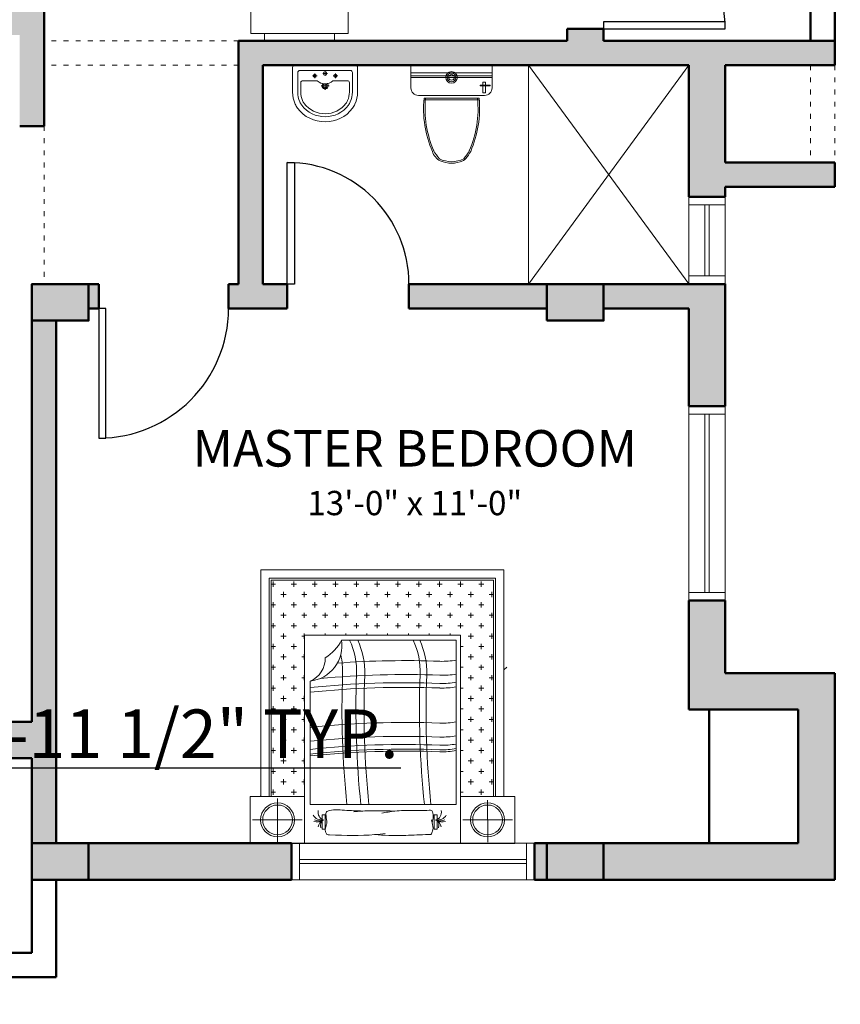
# Model space of a CAD drawing. Units: inches. Extents: x 375 to 1122, y 27 to 1069.
# Tile 67 of 155: x 788 to 990, y 157 to 400. Entities that reach past the tile are written whole.
import ezdxf

# ---------------------------------------------------------------- set-up
doc = ezdxf.new("R2010")
doc.units = ezdxf.units.IN
doc.linetypes.add('ACAD_ISO03W100', pattern=[30, 12, -18])
for name, color, linetype, lineweight in [('A-ANNO-DIMS', 2, 'Continuous', 18), ('A-AREA-IDEN', 7, 'Continuous', 18), ('A-COLS-PATT', 10, 'Continuous', 13), ('A-EQPM', 55, 'Continuous', 18), ('A-FLOR-FIXT', 55, 'Continuous', 18), ('A-WALL-OVHD', 77, 'ACAD_ISO03W100', 18), ('A-WALL-PATT', 252, 'Continuous', 13), ('Columns', 10, 'Continuous', 50), ('Doors', 150, 'Continuous', 25), ('Furniture', 30, 'Continuous', 18), ('Shower Areas', 53, 'Continuous', 18), ('Walls', 250, 'Continuous', 50), ('Windows', 122, 'Continuous', 18)]:
    doc.layers.add(name, color=color, linetype=linetype, lineweight=lineweight)
doc.styles.get("Standard").update_dxf_attribs({"font": 'arial.ttf'})
doc.dimstyles.new('ISO-25', dxfattribs={"dimtxt": 12, "dimasz": 2.5, "dimexe": 1.5, "dimexo": 1.5, "dimtad": 1, "dimdec": 1, "dimlunit": 3, "dimtxsty": 'Standard', "dimblk": 'ARCHTICK', "dimcen": 2.5, "dimadec": 0, "dimazin": 0, "dimtfac": 1, "dimtdec": 1, "dimtmove": 0, "dimatfit": 3, "dimfxl": 1.5, "dimfxlon": 1, "dimarcsym": 0})

# ---------------------------------------------------------------- blocks, each defined once
blk = doc.blocks.new('*U2')
for p, q in [((0, 0), (0, 4)), ((32, 0), (32, 4))]:
    blk.add_line(p, q)
blk.add_lwpolyline([(0, 0), (0, -32), (1.75, -32), (1.75, 0)], close=True)
blk.add_arc((0, 0), 32, 270, 0)
blk = doc.blocks.new('*U3')
for p, q in [((0, 0), (0, -4)), ((30, 0), (30, -4))]:
    blk.add_line(p, q)
blk.add_lwpolyline([(0, 0), (0, 30), (1.75, 30), (1.75, 0)], close=True)
blk.add_arc((0, 0), 30, 0, 90)
blk = doc.blocks.new('*U13')
for p, q in [((-30, 0), (-30, -4)), ((0, 0), (0, -4))]:
    blk.add_line(p, q)
blk.add_lwpolyline([(0, 0), (0, 30), (-1.75, 30), (-1.75, 0)], close=True)
blk.add_arc((0, 0), 30, 90, 180)
blk = doc.blocks.new('A$C52B64FF5')
for p, q in [((0.5216, 2.6276), (0, 2.6276)), ((0, 2.6276), (0, 2.1776)), ((0.2616, 2.4026), (0.2616, 2.6161)), ((0.5216, 2.1776), (0.5216, 2.6276)), ((2.0216, 2.6276), (0.5216, 2.6276)), ((0.5216, 2.6276), (0.5216, 0.6276)), ((2.5432, 2.6276), (2.0216, 2.6276)), ((2.0216, 0.6276), (2.0216, 2.6276)), ((2.0216, 2.6276), (2.0216, 2.1776)), ((2.2816, 2.4026), (2.2816, 2.6161)), ((2.5432, 2.1776), (2.5432, 2.6276)), ((0.721, 2.4927), (0.6917, 2.4927)), ((0.6917, 2.4927), (0.6917, 2.3531)), ((0.721, 2.3531), (0.721, 2.4927)), ((1.767, 2.3531), (1.767, 2.4927)), ((1.767, 2.4927), (1.7964, 2.4927)), ((1.7964, 2.4927), (1.7964, 2.3531)), ((0.2632, 2.4026), (0.0233, 2.4026)), ((0.0233, 2.4026), (0.4999, 2.4026)), ((0.2632, 2.1952), (0.2632, 2.4026)), ((2.5199, 2.4026), (2.0434, 2.4026)), ((2.2801, 2.2128), (2.2801, 2.4026)), ((2.2801, 2.4026), (2.5199, 2.4026)), ((0.6917, 2.3531), (0.721, 2.3531)), ((1.7964, 2.3531), (1.767, 2.3531)), ((0, 2.1776), (0.5216, 2.1776)), ((0.093, 2.1776), (0.1008, 2.1698)), ((0.1008, 0), (0.1008, 2.1776)), ((0.1808, 0.08), (0.1808, 2.1776)), ((0.2008, 0.1), (0.2008, 2.1776)), ((0.5751, 1.0685), (0.5751, 2.2541)), ((0.5751, 2.2541), (1.9782, 2.2541)), ((1.9782, 2.2541), (1.9782, 0.6749)), ((2.5432, 2.1776), (2.0216, 2.1776)), ((2.0216, 2.1776), (2.5432, 2.1776)), ((2.3374, 2.1776), (2.3374, 0.1)), ((2.3574, 2.1776), (2.3574, 0.08)), ((2.4374, 2.1776), (2.4374, 0)), ((0.2008, 2.136), (0.2447, 2.136)), ((0.2197, 2.111), (0.2197, 2.161)), ((0.3947, 2.136), (0.4447, 2.136)), ((0.4197, 2.111), (0.4197, 2.161)), ((2.0216, 2.136), (2.0447, 2.136)), ((2.1947, 2.136), (2.2447, 2.136)), ((2.2197, 2.111), (2.2197, 2.161)), ((0.2947, 2.036), (0.3447, 2.036)), ((0.3197, 2.011), (0.3197, 2.061)), ((0.4947, 2.036), (0.5216, 2.036)), ((0.5197, 2.011), (0.5197, 2.061)), ((2.0947, 2.036), (2.1447, 2.036)), ((2.1197, 2.011), (2.1197, 2.061)), ((2.2947, 2.036), (2.3374, 2.036)), ((2.3197, 2.011), (2.3197, 2.061)), ((0.2008, 1.936), (0.2447, 1.936)), ((0.2197, 1.911), (0.2197, 1.961)), ((0.3947, 1.936), (0.4447, 1.936)), ((0.4197, 1.911), (0.4197, 1.961)), ((2.0216, 1.936), (2.0447, 1.936)), ((2.1947, 1.936), (2.2447, 1.936)), ((2.2197, 1.911), (2.2197, 1.961)), ((0.2947, 1.836), (0.3447, 1.836)), ((0.3197, 1.811), (0.3197, 1.861)), ((0.4947, 1.836), (0.5216, 1.836)), ((0.5197, 1.811), (0.5197, 1.861)), ((2.0947, 1.836), (2.1447, 1.836)), ((2.1197, 1.811), (2.1197, 1.861)), ((2.2947, 1.836), (2.3374, 1.836)), ((2.3197, 1.811), (2.3197, 1.861)), ((0.2008, 1.736), (0.2447, 1.736)), ((0.2197, 1.711), (0.2197, 1.761)), ((0.3947, 1.736), (0.4447, 1.736)), ((0.4197, 1.711), (0.4197, 1.761)), ((2.0216, 1.736), (2.0447, 1.736)), ((2.1947, 1.736), (2.2447, 1.736)), ((2.2197, 1.711), (2.2197, 1.761)), ((0.2947, 1.636), (0.3447, 1.636)), ((0.3197, 1.611), (0.3197, 1.661)), ((0.4947, 1.636), (0.5216, 1.636)), ((0.5197, 1.611), (0.5197, 1.661)), ((2.0947, 1.636), (2.1447, 1.636)), ((2.1197, 1.611), (2.1197, 1.661)), ((2.2947, 1.636), (2.3374, 1.636)), ((2.3197, 1.611), (2.3197, 1.661)), ((0.2008, 1.536), (0.2447, 1.536)), ((0.2197, 1.511), (0.2197, 1.561)), ((0.3947, 1.536), (0.4447, 1.536)), ((0.4197, 1.511), (0.4197, 1.561)), ((2.0216, 1.536), (2.0447, 1.536)), ((2.1947, 1.536), (2.2447, 1.536)), ((2.2197, 1.511), (2.2197, 1.561)), ((0.2947, 1.436), (0.3447, 1.436)), ((0.3197, 1.411), (0.3197, 1.461)), ((0.4947, 1.436), (0.5216, 1.436)), ((0.5197, 1.411), (0.5197, 1.461)), ((2.0947, 1.436), (2.1447, 1.436)), ((2.1197, 1.411), (2.1197, 1.461)), ((2.2947, 1.436), (2.3374, 1.436)), ((2.3197, 1.411), (2.3197, 1.461)), ((0.2008, 1.336), (0.2447, 1.336)), ((0.2197, 1.311), (0.2197, 1.361)), ((0.3947, 1.336), (0.4447, 1.336)), ((0.4197, 1.311), (0.4197, 1.361)), ((2.0216, 1.336), (2.0447, 1.336)), ((2.1947, 1.336), (2.2447, 1.336)), ((2.2197, 1.311), (2.2197, 1.361)), ((0.2947, 1.236), (0.3447, 1.236)), ((0.3197, 1.211), (0.3197, 1.261)), ((0.4947, 1.236), (0.5216, 1.236)), ((0.5197, 1.211), (0.5197, 1.261)), ((2.0947, 1.236), (2.1447, 1.236)), ((2.1197, 1.211), (2.1197, 1.261)), ((2.2947, 1.236), (2.3374, 1.236)), ((2.3197, 1.211), (2.3197, 1.261)), ((0.2008, 1.136), (0.2447, 1.136)), ((0.2197, 1.111), (0.2197, 1.161)), ((0.3947, 1.136), (0.4447, 1.136)), ((0.4197, 1.111), (0.4197, 1.161)), ((2.0216, 1.136), (2.0447, 1.136)), ((2.1947, 1.136), (2.2447, 1.136)), ((2.2197, 1.111), (2.2197, 1.161)), ((0.3197, 1.011), (0.3197, 1.061)), ((0.5197, 1.011), (0.5197, 1.061)), ((2.1197, 1.011), (2.1197, 1.061)), ((2.3197, 1.011), (2.3197, 1.061)), ((0.2197, 0.911), (0.2197, 0.961)), ((0.2947, 1.036), (0.3447, 1.036)), ((0.4197, 0.911), (0.4197, 0.961)), ((0.4947, 1.036), (0.5216, 1.036)), ((2.0947, 1.036), (2.1447, 1.036)), ((2.2197, 0.911), (2.2197, 0.961)), ((2.2947, 1.036), (2.3374, 1.036)), ((2.4374, 0.9617), (2.4642, 0.935)), ((0.2008, 0.936), (0.2447, 0.936)), ((0.3197, 0.811), (0.3197, 0.861)), ((0.3947, 0.936), (0.4447, 0.936)), ((0.5197, 0.811), (0.5197, 0.861)), ((2.0216, 0.936), (2.0447, 0.936)), ((2.1197, 0.811), (2.1197, 0.861)), ((2.1947, 0.936), (2.2447, 0.936)), ((2.3197, 0.811), (2.3197, 0.861)), ((0.2197, 0.711), (0.2197, 0.761)), ((0.2947, 0.836), (0.3447, 0.836)), ((0.4197, 0.711), (0.4197, 0.761)), ((0.4947, 0.836), (0.5216, 0.836)), ((2.0947, 0.836), (2.1447, 0.836)), ((2.2197, 0.711), (2.2197, 0.761)), ((2.2947, 0.836), (2.3374, 0.836)), ((0.2008, 0.736), (0.2447, 0.736)), ((0.3947, 0.736), (0.4447, 0.736)), ((1.9782, 0.6749), (0.8764, 0.6749)), ((2.0216, 0.736), (2.0447, 0.736)), ((2.1947, 0.736), (2.2447, 0.736)), ((0.2947, 0.636), (0.3447, 0.636)), ((0.3197, 0.611), (0.3197, 0.661)), ((0.4947, 0.636), (0.5216, 0.636)), ((0.5197, 0.611), (0.5197, 0.661)), ((0.5216, 0.6276), (2.0216, 0.6276)), ((0.7197, 0.611), (0.7197, 0.6276)), ((0.9197, 0.611), (0.9197, 0.6276)), ((1.1197, 0.611), (1.1197, 0.6276)), ((1.3197, 0.611), (1.3197, 0.6276)), ((1.5197, 0.611), (1.5197, 0.6276)), ((1.7197, 0.611), (1.7197, 0.6276)), ((1.9197, 0.611), (1.9197, 0.6276)), ((2.0947, 0.636), (2.1447, 0.636)), ((2.1197, 0.611), (2.1197, 0.661)), ((2.2947, 0.636), (2.3374, 0.636)), ((2.3197, 0.611), (2.3197, 0.661)), ((0.2008, 0.536), (0.2447, 0.536)), ((0.2197, 0.511), (0.2197, 0.561)), ((0.3947, 0.536), (0.4447, 0.536)), ((0.4197, 0.511), (0.4197, 0.561)), ((0.5947, 0.536), (0.6447, 0.536)), ((0.6197, 0.511), (0.6197, 0.561)), ((0.7947, 0.536), (0.8447, 0.536)), ((0.8197, 0.511), (0.8197, 0.561)), ((0.9947, 0.536), (1.0447, 0.536)), ((1.0197, 0.511), (1.0197, 0.561)), ((1.1947, 0.536), (1.2447, 0.536)), ((1.2197, 0.511), (1.2197, 0.561)), ((1.3947, 0.536), (1.4447, 0.536)), ((1.4197, 0.511), (1.4197, 0.561)), ((1.5947, 0.536), (1.6447, 0.536)), ((1.6197, 0.511), (1.6197, 0.561)), ((1.7947, 0.536), (1.8447, 0.536)), ((1.8197, 0.511), (1.8197, 0.561)), ((1.9947, 0.536), (2.0447, 0.536)), ((2.0197, 0.511), (2.0197, 0.561)), ((2.1947, 0.536), (2.2447, 0.536)), ((2.2197, 0.511), (2.2197, 0.561)), ((0.2947, 0.436), (0.3447, 0.436)), ((0.3197, 0.411), (0.3197, 0.461)), ((0.4947, 0.436), (0.5447, 0.436)), ((0.5197, 0.411), (0.5197, 0.461)), ((0.6947, 0.436), (0.7447, 0.436)), ((0.7197, 0.411), (0.7197, 0.461)), ((0.8947, 0.436), (0.9447, 0.436)), ((0.9197, 0.411), (0.9197, 0.461)), ((1.0947, 0.436), (1.1447, 0.436)), ((1.1197, 0.411), (1.1197, 0.461)), ((1.2947, 0.436), (1.3447, 0.436)), ((1.3197, 0.411), (1.3197, 0.461)), ((1.4947, 0.436), (1.5447, 0.436)), ((1.5197, 0.411), (1.5197, 0.461)), ((1.6947, 0.436), (1.7447, 0.436)), ((1.7197, 0.411), (1.7197, 0.461)), ((1.8947, 0.436), (1.9447, 0.436)), ((1.9197, 0.411), (1.9197, 0.461)), ((2.0947, 0.436), (2.1447, 0.436)), ((2.1197, 0.411), (2.1197, 0.461)), ((2.2947, 0.436), (2.3374, 0.436)), ((2.3197, 0.411), (2.3197, 0.461)), ((0.2008, 0.336), (0.2447, 0.336)), ((0.2197, 0.311), (0.2197, 0.361)), ((0.3947, 0.336), (0.4447, 0.336)), ((0.4197, 0.311), (0.4197, 0.361)), ((0.5947, 0.336), (0.6447, 0.336)), ((0.6197, 0.311), (0.6197, 0.361)), ((0.7947, 0.336), (0.8447, 0.336)), ((0.8197, 0.311), (0.8197, 0.361)), ((0.9947, 0.336), (1.0447, 0.336)), ((1.0197, 0.311), (1.0197, 0.361)), ((1.1947, 0.336), (1.2447, 0.336)), ((1.2197, 0.311), (1.2197, 0.361)), ((1.3947, 0.336), (1.4447, 0.336)), ((1.4197, 0.311), (1.4197, 0.361)), ((1.5947, 0.336), (1.6447, 0.336)), ((1.6197, 0.311), (1.6197, 0.361)), ((1.7947, 0.336), (1.8447, 0.336)), ((1.8197, 0.311), (1.8197, 0.361)), ((1.9947, 0.336), (2.0447, 0.336)), ((2.0197, 0.311), (2.0197, 0.361)), ((2.1947, 0.336), (2.2447, 0.336)), ((2.2197, 0.311), (2.2197, 0.361)), ((0.2947, 0.236), (0.3447, 0.236)), ((0.3197, 0.211), (0.3197, 0.261)), ((0.4947, 0.236), (0.5447, 0.236)), ((0.5197, 0.211), (0.5197, 0.261)), ((0.6947, 0.236), (0.7447, 0.236)), ((0.7197, 0.211), (0.7197, 0.261)), ((0.8947, 0.236), (0.9447, 0.236)), ((0.9197, 0.211), (0.9197, 0.261)), ((1.0947, 0.236), (1.1447, 0.236)), ((1.1197, 0.211), (1.1197, 0.261)), ((1.2947, 0.236), (1.3447, 0.236)), ((1.3197, 0.211), (1.3197, 0.261)), ((1.4947, 0.236), (1.5447, 0.236)), ((1.5197, 0.211), (1.5197, 0.261)), ((1.6947, 0.236), (1.7447, 0.236)), ((1.7197, 0.211), (1.7197, 0.261)), ((1.8947, 0.236), (1.9447, 0.236)), ((1.9197, 0.211), (1.9197, 0.261)), ((2.0947, 0.236), (2.1447, 0.236)), ((2.1197, 0.211), (2.1197, 0.261)), ((2.2947, 0.236), (2.3374, 0.236)), ((2.3197, 0.211), (2.3197, 0.261)), ((0.2008, 0.136), (0.2447, 0.136)), ((2.3374, 0.1), (0.2008, 0.1)), ((0.2197, 0.111), (0.2197, 0.161)), ((0.3947, 0.136), (0.4447, 0.136)), ((0.4197, 0.111), (0.4197, 0.161)), ((0.5947, 0.136), (0.6447, 0.136)), ((0.6197, 0.111), (0.6197, 0.161)), ((0.7947, 0.136), (0.8447, 0.136)), ((0.8197, 0.111), (0.8197, 0.161)), ((0.9947, 0.136), (1.0447, 0.136)), ((1.0197, 0.111), (1.0197, 0.161)), ((1.1947, 0.136), (1.2447, 0.136)), ((1.2197, 0.111), (1.2197, 0.161)), ((1.3947, 0.136), (1.4447, 0.136)), ((1.4197, 0.111), (1.4197, 0.161)), ((1.5947, 0.136), (1.6447, 0.136)), ((1.6197, 0.111), (1.6197, 0.161)), ((1.7947, 0.136), (1.8447, 0.136)), ((1.8197, 0.111), (1.8197, 0.161)), ((1.9947, 0.136), (2.0447, 0.136)), ((2.0197, 0.111), (2.0197, 0.161)), ((2.1947, 0.136), (2.2447, 0.136)), ((2.2197, 0.111), (2.2197, 0.161)), ((2.4374, 0), (0.1008, 0)), ((2.3574, 0.08), (0.1808, 0.08))]:
    blk.add_line(p, q)
for centre, radius in [((0.2632, 2.4026), 0.1631), ((2.2801, 2.4026), 0.1631), ((0.2632, 2.4026), 0.1431), ((2.2801, 2.4026), 0.1431)]:
    blk.add_circle(centre, radius)
for centre, radius, start, end in [((0.7523, 2.4916), 0.1013, 192.77399, 239.2386), ((0.7566, 2.4523), 0.0808, 161.45592, 221.5545), ((1.7358, 2.4916), 0.1013, 300.7614, 347.22601), ((1.7315, 2.4523), 0.0808, 318.4455, 18.54408), ((0.6895, 2.3063), 0.098, 80.94857, 149.48786), ((0.6442, 2.3154), 0.1072, 59.2174, 107.24009), ((0.6646, 2.3215), 0.0913, 67.83977, 120.48585), ((0.7294, 2.33), 0.0776, 109.26419, 192.26691), ((1.7587, 2.33), 0.0776, 347.73309, 73.88358), ((1.7986, 2.3063), 0.098, 30.51214, 99.05143), ((1.8439, 2.3154), 0.1072, 72.75991, 120.7826), ((1.8235, 2.3215), 0.0913, 59.51415, 112.16023), ((9.7293, 1.3409), 8.8479, 174.07538, 182.16616), ((9.8633, 1.3409), 8.8479, 174.07538, 182.16616), ((9.9414, 1.3409), 8.8479, 174.07538, 182.16616), ((10.4736, 1.3409), 8.8479, 174.07538, 182.16616), ((10.5369, 1.3409), 8.8479, 174.07538, 182.16616), ((1.4884, 10.5889), 8.8479, 264.07538, 272.16616), ((1.4884, 10.5702), 8.8479, 264.07538, 272.16616), ((1.4884, 10.5256), 8.8479, 264.07538, 272.16616), ((1.85, 1.0282), 0.7196, 79.7409, 92.16616), ((1.85, 1.0096), 0.7196, 79.7409, 92.16616), ((1.4884, 10.4474), 8.8479, 264.07538, 272.16616), ((1.85, 0.965), 0.7196, 79.7409, 92.16616), ((1.85, 0.8868), 0.7196, 79.7409, 92.16616), ((1.4884, 10.3135), 8.8479, 264.07538, 272.16616), ((1.85, 0.7528), 0.7196, 79.7409, 92.16616), ((1.4884, 9.9764), 8.8479, 264.07538, 272.16616), ((1.4884, 9.9317), 8.8479, 264.07538, 272.16616), ((0.4865, 0.8516), 0.2343, 358.03681, 67.7864), ((0.5391, 0.7288), 0.3416, 350.92672, 83.95649), ((1.4884, 9.8536), 8.8479, 264.70583, 272.16616), ((1.85, 0.4158), 0.7196, 79.7409, 92.16616), ((1.85, 0.3711), 0.7196, 79.7409, 92.16616), ((0.1687, 0.9792), 0.7196, 346.86533, 2.16616), ((0.3027, 0.9792), 0.7196, 334.98359, 2.16616), ((0.3808, 0.9792), 0.7196, 334.98359, 2.16616), ((0.913, 0.9792), 0.7196, 334.98359, 2.16616), ((0.9763, 0.9792), 0.7196, 334.98359, 2.16616), ((1.85, 0.293), 0.7196, 79.7409, 92.16616), ((1.4884, 9.7196), 8.8479, 265.77852, 272.16616), ((1.85, 0.159), 0.7196, 79.7409, 92.16616), ((0.5285, 0.5098), 0.3852, 25.3912, 60.06861)]:
    blk.add_arc(centre, radius, start, end)
for points, knots in [([(0.7373, 2.4293), (0.7344, 2.4386), (0.7239, 2.472), (0.715, 2.518), (0.7414, 2.5459), (0.9088, 2.5514), (1.0864, 2.5586), (1.2642, 2.5365), (1.2976, 2.5323)], [0, 0, 0, 0, 0.0298664, 0.1071619, 0.1152509, 0.1416099, 0.5761797, 0.6768951, 0.6768951, 0.6768951, 0.6768951]), ([(1.1947, 2.5438), (1.2853, 2.549), (1.4483, 2.5585), (1.6283, 2.5432), (1.7179, 2.5437), (1.7351, 2.5438)], [0, 0, 0, 0, 0.2717358, 0.4891854, 0.5406465, 0.5406465, 0.5406465, 0.5406465]), ([(1.7351, 2.5438), (1.7416, 2.5321), (1.759, 2.5014), (1.7583, 2.4623), (1.7348, 2.3817), (1.7455, 2.4145), (1.7494, 2.4265)], [0, 0, 0, 0, 0.0383771, 0.1013156, 0.1484959, 0.1756343, 0.1756343, 0.1756343, 0.1756343]), ([(1.0802, 2.3175), (1.0225, 2.3155), (0.9099, 2.3116), (0.7905, 2.2985), (0.7234, 2.3279), (0.7309, 2.3766), (0.7348, 2.4091), (0.7373, 2.4293)], [0, 0, 0, 0, 0.1744349, 0.3406483, 0.347042, 0.3874998, 0.4538558, 0.4538558, 0.4538558, 0.4538558]), ([(1.7494, 2.4265), (1.7531, 2.4084), (1.7601, 2.3751), (1.7573, 2.3363), (1.7437, 2.3065), (1.6676, 2.315), (1.559, 2.3108), (1.4028, 2.3119), (1.305, 2.3301), (1.2633, 2.3378)], [0, 0, 0, 0, 0.0550284, 0.1011576, 0.1178362, 0.1437253, 0.3009935, 0.4726259, 0.6000038, 0.6000038, 0.6000038, 0.6000038]), ([(1.3748, 2.3178), (1.2947, 2.315), (1.1678, 2.3105), (1.0413, 2.32), (0.9946, 2.3235)], [0, 0, 0, 0, 0.2401688, 0.38052, 0.38052, 0.38052, 0.38052])]:
    blk.add_open_spline(points, degree=3, knots=knots)
blk = doc.blocks.new('A$C659B0DF6')
for p, q in [((17.35, 607.55), (17.35, 606.07)), ((21.05, 607.55), (17.35, 607.55)), ((21.05, 606.07), (21.05, 607.55)), ((24, 606.07), (0, 606.07)), ((0, 585.72), (0, 606.07)), ((24, 585.72), (24, 606.07)), ((24, 604.22), (0, 604.22)), ((24, 585.72), (0, 585.72)), ((3.37, 583.91), (3.37, 585.72)), ((20.63, 583.91), (20.63, 585.72)), ((3.37, 583.91), (20.63, 583.91))]:
    blk.add_line(p, q)
blk = doc.blocks.new('A$C00C51FE0')
at = {"ltscale": 2}
for p, q in [((1.85, 7.41), (18.15, 7.41)), ((16.79, 8.49), (3.21, 8.49)), ((16.79, 8.12), (3.21, 8.12)), ((0, 0), (0, 5.56)), ((0.5, 4.84), (0.5, 5.06)), ((0.5, 5.06), (2.91, 5.06)), ((1.59, 4.18), (1.59, 6.81)), ((1.59, 6.81), (2.25, 6.81)), ((2.25, 6.81), (2.25, 4.18)), ((2.91, 5.06), (2.91, 4.84)), ((20, 5.56), (20, 0)), ((20, 2.96), (0, 2.96)), ((20, 2.59), (0, 2.59)), ((2.91, 4.84), (0.5, 4.84)), ((2.25, 4.18), (1.59, 4.18)), ((20, 1.85), (0, 1.85)), ((20, 0), (0, 0))]:
    blk.add_line(p, q, dxfattribs=at)
for radius in [1.44, 1.07, 0.698]:
    blk.add_circle((10, 2.96), radius, dxfattribs=at)
for centre, radius, start, end in [((22.68, 10.69), 20.34, 142.816, 148.8373), ((22.68, 10.69), 19.97, 141.7352, 148.8373), ((7.96, 21.86), 1.85, 112.9199, 142.816), ((10, 17.03), 6.73, 63.5839, 116.4161), ((10, 17.03), 7.1, 67.0801, 112.9199), ((11.04, 20.15), 3.83, 16.1902, 63.2078), ((-2.68, 10.69), 19.97, 31.1627, 38.2648), ((29.69, 10.65), 26.6, 156.5869, 185.4494), ((29.69, 10.65), 26.23, 156.5869, 185.4494), ((-9.69, 10.65), 26.23, 354.5506, 23.4131), ((-9.69, 10.65), 26.6, 354.5506, 23.4131), ((1.85, 5.56), 1.85, 90, 180), ((18.15, 5.56), 1.85, 0, 90)]:
    blk.add_arc(centre, radius, start, end, dxfattribs=at)
blk = doc.blocks.new('WINDOW-48IN')
for p, q in [((2, 5), (46, 5)), ((2, 4), (46, 4))]:
    blk.add_line(p, q)
blk.add_lwpolyline([(48, 0), (0, 0), (0, 9), (48, 9)], close=True)
for points in [[(2, 0), (2, 9)], [(46, 9), (46, 0)]]:
    blk.add_lwpolyline(points)
blk = doc.blocks.new('WINDOW-21_5IN')
for p, q in [((4, 2), (4, 19.5)), ((5, 2), (5, 19.5))]:
    blk.add_line(p, q)
blk.add_lwpolyline([(0, 0), (9, 0), (9, 21.5), (0, 21.5)], close=True)
for points in [[(9, 19.5), (0, 19.5)], [(0, 2), (9, 2)]]:
    blk.add_lwpolyline(points)
blk = doc.blocks.new('WINDOW-60IN')
for p, q in [((58, 5), (2, 5)), ((58, 4), (2, 4))]:
    blk.add_line(p, q)
blk.add_lwpolyline([(60, 0), (0, 0), (0, 9), (60, 9)], close=True)
for points in [[(2, 0), (2, 9)], [(58, 9), (58, 0)]]:
    blk.add_lwpolyline(points)
blk = doc.blocks.new('LAVATORY-16IN')
for p, q in [((1.27, 7.37), (1.27, 12.19)), ((1.78, 12.7), (14.22, 12.7)), ((8, 11.37), (8, 12.51)), ((14.73, 12.19), (14.73, 7.37)), ((2.51, 10.16), (6.08, 10.16)), ((4.89, 11.37), (6.03, 11.37)), ((5.46, 10.79), (5.46, 11.94)), ((7.43, 11.94), (8.57, 11.94)), ((9.91, 10.16), (13.49, 10.16)), ((9.97, 11.37), (11.11, 11.37)), ((10.54, 10.79), (10.54, 11.94)), ((2.01, 7.37), (2.01, 9.65)), ((7.02, 8.89), (8.98, 8.89)), ((8, 7.91), (8, 9.4)), ((13.99, 9.65), (13.99, 7.37))]:
    blk.add_line(p, q)
blk.add_lwpolyline([(0.51, 13.97), (15.49, 13.97, -0.414214), (16, 13.46), (16, 7.37, -0.104704), (15.37, 4.36, -0.038376), (14.78, 3.36, -0.495903), (1.22, 3.36, -0.038376), (0.63, 4.36, -0.104704), (0, 7.37), (0, 13.46, -0.414214)], format="xyb", close=True)
for points in [[(1.27, 7.37, 0.102694), (1.78, 4.92, 0.037256), (2.25, 4.11, 0.085618)], [(2.01, 7.37, 0.101044), (2.44, 5.24, 0.036381), (2.84, 4.54, 0.084644)], [(13.16, 4.54, 0.036381), (13.56, 5.24, 0.101044), (13.99, 7.37, 0.11083)], [(13.75, 4.11, 0.037256), (14.22, 4.92, 0.102694), (14.73, 7.37, 0.111333)]]:
    blk.add_lwpolyline(points, format="xyb")
for centre, radius in [((8, 11.94), 0.444), ((5.46, 11.37), 0.381), ((10.54, 11.37), 0.381), ((8, 8.89), 0.508)]:
    blk.add_circle(centre, radius)
for centre, radius, start, end in [((1.78, 12.19), 0.508, 90, 180), ((14.22, 12.19), 0.508, 0, 90), ((2.51, 9.65), 0.508, 90, 180), ((7.99, 12.19), 2.79, 226.6581, 313.3419), ((13.49, 9.65), 0.508, 0, 90), ((8, 8.89), 0.762, 133.135, 47.0367), ((8, 8.52), 7.25, 217.471, 322.529), ((8, 8.52), 6.51, 217.6433, 322.3567)]:
    blk.add_arc(centre, radius, start, end)
blk = doc.blocks.new('COLUMN-14X9IN')
blk.add_lwpolyline([(0, 0), (14, 0), (14, 9), (0, 9)], close=True)
blk = doc.blocks.new('SHOWER-PAN-39_5X54IN')
for p, q in [((0, 0), (39.5, 54)), ((0, 54), (39.5, 0.05))]:
    blk.add_line(p, q)
blk.add_lwpolyline([(39.5, 54), (0, 54), (0, 0), (39.5, 0)], close=True)
blk = doc.blocks.new('_ArchTick')
at = {"color": 0, "linetype": 'ByBlock', "const_width": 0.15}
blk.add_lwpolyline([(-0.5, -0.5), (0.5, 0.5)], dxfattribs=at)
blk = doc.blocks.new('*D60')
at = {"layer": 'A-ANNO-DIMS', "color": 0, "lineweight": -2, "transparency": 16777216}
for p, q in [((684.39, 216.67), (684.39, 213.67)), ((767.77, 216.67), (767.77, 213.67)), ((684.39, 215.17), (767.77, 215.17)), ((767.77, 215.17), (882.02, 215.17))]:
    blk.add_line(p, q, dxfattribs=at)
at = {"layer": 'Defpoints', "color": 0, "transparency": 16777216}
for p in [(684.39, 232.35), (767.77, 232.35), (767.77, 215.17)]:
    blk.add_point(p, dxfattribs=at)
at = {"layer": 'A-ANNO-DIMS', "color": 0, "lineweight": -2, "transparency": 16777216, "xscale": 2.5, "yscale": 2.5, "zscale": 2.5, "rotation": 180}
blk.add_blockref('_ArchTick', (684.39, 215.17), dxfattribs=at)
at = {"layer": 'A-ANNO-DIMS', "color": 0, "lineweight": -2, "transparency": 16777216, "xscale": 2.5, "yscale": 2.5, "zscale": 2.5}
blk.add_blockref('_ArchTick', (767.77, 215.17), dxfattribs=at)
at = {"layer": 'A-ANNO-DIMS', "color": 0, "transparency": 16777216, "insert": (826.15, 222), "char_height": 12, "attachment_point": 5}
blk.add_mtext('6\'-11 1/2" TYP.', dxfattribs=at)
blk = doc.blocks.new('*D81')
at = {"layer": 'A-ANNO-DIMS', "color": 0, "lineweight": -2, "transparency": 16777216}
for p, q in [((444.51, 117.53), (444.51, 114.53)), ((989.01, 117.53), (989.01, 114.53)), ((444.51, 116.03), (989.01, 116.03))]:
    blk.add_line(p, q, dxfattribs=at)
at = {"layer": 'Defpoints', "color": 0, "transparency": 16777216}
for p in [(444.51, 187.53), (989.01, 187.53), (989.01, 116.03)]:
    blk.add_point(p, dxfattribs=at)
at = {"layer": 'A-ANNO-DIMS', "color": 0, "lineweight": -2, "transparency": 16777216, "xscale": 2.5, "yscale": 2.5, "zscale": 2.5, "rotation": 180}
blk.add_blockref('_ArchTick', (444.51, 116.03), dxfattribs=at)
at = {"layer": 'A-ANNO-DIMS', "color": 0, "lineweight": -2, "transparency": 16777216, "xscale": 2.5, "yscale": 2.5, "zscale": 2.5}
blk.add_blockref('_ArchTick', (989.01, 116.03), dxfattribs=at)
at = {"layer": 'A-ANNO-DIMS', "color": 0, "transparency": 16777216, "insert": (716.76, 122.86), "char_height": 12, "attachment_point": 5}
blk.add_mtext('45\'-4 1/2"', dxfattribs=at)
blk = doc.blocks.new('*D84')
at = {"layer": 'A-ANNO-DIMS', "color": 0, "lineweight": -2, "transparency": 16777216}
for p, q in [((845.01, 117.53), (845.01, 114.53)), ((950.01, 117.53), (950.01, 114.53)), ((845.01, 116.03), (950.01, 116.03))]:
    blk.add_line(p, q, dxfattribs=at)
at = {"layer": 'Defpoints', "color": 0, "transparency": 16777216}
for p in [(845.01, 814.53), (950.01, 814.53), (950.01, 116.03)]:
    blk.add_point(p, dxfattribs=at)
at = {"layer": 'A-ANNO-DIMS', "color": 0, "lineweight": -2, "transparency": 16777216, "xscale": 2.5, "yscale": 2.5, "zscale": 2.5, "rotation": 180}
blk.add_blockref('_ArchTick', (845.01, 116.03), dxfattribs=at)
at = {"layer": 'A-ANNO-DIMS', "color": 0, "lineweight": -2, "transparency": 16777216, "xscale": 2.5, "yscale": 2.5, "zscale": 2.5}
blk.add_blockref('_ArchTick', (950.01, 116.03), dxfattribs=at)
at = {"layer": 'A-ANNO-DIMS', "color": 0, "transparency": 16777216, "insert": (897.51, 122.78), "char_height": 12, "attachment_point": 5}
blk.add_mtext('8\'-9"', dxfattribs=at)
blk = doc.blocks.new('*D87')
at = {"layer": 'A-ANNO-DIMS', "color": 0, "lineweight": -2, "transparency": 16777216}
for p, q in [((794.01, 117.53), (794.01, 114.53)), ((884.01, 117.53), (884.01, 114.53)), ((794.01, 116.03), (884.01, 116.03))]:
    blk.add_line(p, q, dxfattribs=at)
at = {"layer": 'Defpoints', "color": 0, "transparency": 16777216}
for p in [(794.01, 583.53), (884.01, 583.53), (884.01, 116.03)]:
    blk.add_point(p, dxfattribs=at)
at = {"layer": 'A-ANNO-DIMS', "color": 0, "lineweight": -2, "transparency": 16777216, "xscale": 2.5, "yscale": 2.5, "zscale": 2.5, "rotation": 180}
blk.add_blockref('_ArchTick', (794.01, 116.03), dxfattribs=at)
at = {"layer": 'A-ANNO-DIMS', "color": 0, "lineweight": -2, "transparency": 16777216, "xscale": 2.5, "yscale": 2.5, "zscale": 2.5}
blk.add_blockref('_ArchTick', (884.01, 116.03), dxfattribs=at)
at = {"layer": 'A-ANNO-DIMS', "color": 0, "transparency": 16777216, "insert": (839.01, 122.78), "char_height": 12, "attachment_point": 5}
blk.add_mtext('7\'-6"', dxfattribs=at)
blk = doc.blocks.new('*D89')
at = {"layer": 'A-ANNO-DIMS', "color": 0, "lineweight": -2, "transparency": 16777216}
for p, q in [((863.01, 117.53), (863.01, 114.53)), ((923.01, 117.53), (923.01, 114.53)), ((863.01, 116.03), (923.01, 116.03))]:
    blk.add_line(p, q, dxfattribs=at)
at = {"layer": 'Defpoints', "color": 0, "transparency": 16777216}
for p in [(863.01, 574.53), (923.01, 574.53), (923.01, 116.03)]:
    blk.add_point(p, dxfattribs=at)
at = {"layer": 'A-ANNO-DIMS', "color": 0, "lineweight": -2, "transparency": 16777216, "xscale": 2.5, "yscale": 2.5, "zscale": 2.5, "rotation": 180}
blk.add_blockref('_ArchTick', (863.01, 116.03), dxfattribs=at)
at = {"layer": 'A-ANNO-DIMS', "color": 0, "lineweight": -2, "transparency": 16777216, "xscale": 2.5, "yscale": 2.5, "zscale": 2.5}
blk.add_blockref('_ArchTick', (923.01, 116.03), dxfattribs=at)
at = {"layer": 'A-ANNO-DIMS', "color": 0, "transparency": 16777216, "insert": (893.01, 122.78), "char_height": 12, "attachment_point": 5}
blk.add_mtext('5\'-0"', dxfattribs=at)

msp = doc.modelspace()

# ---------------------------------------------------------------- hatches: boundary and pattern name
at = {"layer": 'A-COLS-PATT'}
h = msp.add_hatch(color=256, dxfattribs=at)
h.dxf.hatch_style = 1
h.paths.add_polyline_path([(512.51, 982.53), (498.51, 982.53), (498.51, 973.53), (512.51, 973.53)])
h.paths.add_polyline_path([(666.51, 982.53), (652.51, 982.53), (652.51, 973.53), (666.51, 973.53)])
h.paths.add_polyline_path([(802.01, 982.53), (788.01, 982.53), (788.01, 973.53), (802.01, 973.53)])
h.paths.add_polyline_path([(932.01, 982.53), (918.01, 982.53), (918.01, 973.53), (932.01, 973.53)])
h.paths.add_polyline_path([(507.51, 841.53), (498.51, 841.53), (498.51, 827.53), (507.51, 827.53)])
h.paths.add_polyline_path([(666.51, 844.53), (652.51, 844.53), (652.51, 835.53), (666.51, 835.53)])
h.paths.add_polyline_path([(802.01, 814.53), (788.01, 814.53), (788.01, 805.53), (802.01, 805.53)])
h.paths.add_polyline_path([(932.01, 814.53), (918.01, 814.53), (918.01, 805.53), (932.01, 805.53)])
h.paths.add_polyline_path([(507.51, 719.53), (498.51, 719.53), (498.51, 705.53), (507.51, 705.53)])
h.paths.add_polyline_path([(731.01, 676.53), (722.01, 676.53), (722.01, 662.53), (731.01, 662.53)])
h.paths.add_polyline_path([(802.01, 676.53), (788.01, 676.53), (788.01, 667.53), (802.01, 667.53)])
h.paths.add_polyline_path([(932.01, 676.53), (918.01, 676.53), (918.01, 667.53), (932.01, 667.53)])
h.paths.add_polyline_path([(932.01, 583.53), (918.01, 583.53), (918.01, 574.53), (932.01, 574.53)])
h.paths.add_polyline_path([(868.01, 583.53), (854.01, 583.53), (854.01, 574.53), (868.01, 574.53)])
h.paths.add_polyline_path([(868.01, 502.53), (854.01, 502.53), (854.01, 493.53), (868.01, 493.53)])
h.paths.add_polyline_path([(932.01, 502.53), (918.01, 502.53), (918.01, 493.53), (932.01, 493.53)])
h.paths.add_polyline_path([(672.51, 592.03), (663.51, 592.03), (663.51, 578.03), (672.51, 578.03)])
h.paths.add_polyline_path([(512.51, 589.53), (498.51, 589.53), (498.51, 580.53), (512.51, 580.53)])
h.paths.add_polyline_path([(507.51, 464.53), (498.51, 464.53), (498.51, 450.53), (507.51, 450.53)])
h.paths.add_polyline_path([(731.01, 507.53), (722.01, 507.53), (722.01, 493.53), (731.01, 493.53)])
h.paths.add_polyline_path([(802.01, 502.53), (788.01, 502.53), (788.01, 493.53), (802.01, 493.53)])
h.paths.add_polyline_path([(507.51, 342.53), (498.51, 342.53), (498.51, 328.53), (507.51, 328.53)])
h.paths.add_polyline_path([(512.51, 196.53), (498.51, 196.53), (498.51, 187.53), (512.51, 187.53)])
h.paths.add_polyline_path([(666.51, 334.53), (652.51, 334.53), (652.51, 325.53), (666.51, 325.53)])
h.paths.add_polyline_path([(666.51, 196.53), (652.51, 196.53), (652.51, 187.53), (666.51, 187.53)])
h.paths.add_polyline_path([(805.01, 196.53), (791.01, 196.53), (791.01, 187.53), (805.01, 187.53)])
h.paths.add_polyline_path([(932.01, 196.53), (918.01, 196.53), (918.01, 187.53), (932.01, 187.53)])
h.paths.add_polyline_path([(932.01, 334.53), (918.01, 334.53), (918.01, 325.53), (932.01, 325.53)])
h.paths.add_polyline_path([(805.01, 334.53), (791.01, 334.53), (791.01, 325.53), (805.01, 325.53)])
at = {"layer": 'A-WALL-PATT'}
h = msp.add_hatch(color=256, dxfattribs=at)
h.dxf.hatch_style = 1
h.paths.add_polyline_path([(962.01, 388.53), (989.01, 388.53), (989.01, 394.53), (962.01, 394.53), (932.01, 394.53), (932.01, 397.53), (923.01, 397.53), (923.01, 394.53), (842.01, 394.53), (842.01, 334.53), (839.51, 334.53), (839.51, 328.53), (854.01, 328.53), (854.01, 334.53), (848.01, 334.53), (848.01, 388.53), (953.01, 388.53), (953.01, 356.08), (962.01, 356.08), (962.01, 358.55), (989.01, 358.55), (989.01, 364.55), (962.01, 364.55)])
h.paths.add_polyline_path([(989.01, 502.53), (932.01, 502.53), (932.01, 583.53), (932.01, 593.53), (923.01, 593.53), (923.01, 583.53), (854.01, 583.53), (854.01, 556.53), (863.01, 556.53), (863.01, 574.53), (923.01, 574.53), (923.01, 502.53), (863.01, 502.53), (863.01, 520.53), (854.01, 520.53), (854.01, 502.53), (773.01, 502.53), (773.01, 493.53), (788.01, 493.53), (788.01, 402.03), (722.01, 402.03), (722.01, 373.53), (728.01, 373.53), (728.01, 396.03), (788.01, 396.03), (788.01, 373.53), (794.01, 373.53), (794.01, 430.53), (814.01, 430.53), (814.01, 436.53), (794.01, 436.53), (794.01, 493.53), (923.01, 493.53), (923.01, 487.53), (932.01, 487.53), (932.01, 493.53), (983.01, 493.53), (983.01, 473.53), (989.01, 473.53)])
h.paths.add_polyline_path([(797.01, 325.53), (805.01, 325.53), (805.01, 328.53), (807.51, 328.53), (807.51, 334.53), (791.01, 334.53), (791.01, 226.53), (770.76, 226.53), (770.76, 217.53), (791.01, 217.53), (791.01, 187.53), (855.01, 187.53), (855.01, 196.53), (797.01, 196.53)])
h.paths.add_polyline_path([(989.01, 238.53), (962.01, 238.53), (962.01, 256.42), (953.01, 256.42), (953.01, 229.53), (980.01, 229.53), (980.01, 196.53), (915.01, 196.53), (915.01, 187.53), (989.01, 187.53)])
h.paths.add_polyline_path([(962.01, 334.53), (884.01, 334.53), (884.01, 328.53), (918.01, 328.53), (918.01, 325.53), (932.01, 325.53), (932.01, 328.53), (953.01, 328.53), (953.01, 304.42), (962.01, 304.42)])
h.paths.add_polyline_path([(606.51, 283.53), (609.51, 283.53), (609.51, 289.53), (600.51, 289.53), (600.51, 196.53), (578.51, 196.53), (578.51, 187.53), (606.51, 187.53), (606.51, 196.53)])
h.paths.add_polyline_path([(666.51, 292.53), (660.51, 292.53), (660.51, 289.53), (633.51, 289.53), (633.51, 283.53), (660.51, 283.53), (660.51, 196.53), (628.01, 196.53), (628.01, 187.53), (630.53, 187.53), (630.53, 160.53), (636.53, 160.53), (636.53, 187.53), (660.51, 187.53), (660.51, 160.53), (666.51, 160.53), (666.51, 217.53), (686.76, 217.53), (686.76, 226.53), (666.51, 226.53)])
h.paths.add_polyline_path([(480.51, 256.42), (471.51, 256.42), (471.51, 238.53), (444.51, 238.53), (444.51, 187.53), (518.51, 187.53), (518.51, 196.53), (453.51, 196.53), (453.51, 229.53), (480.51, 229.53)])
h.paths.add_polyline_path([(480.51, 328.53), (652.51, 328.53), (652.51, 325.53), (660.51, 325.53), (660.51, 322.53), (666.51, 322.53), (666.51, 334.53), (507.51, 334.53), (507.51, 360.53), (498.51, 360.53), (498.51, 334.53), (471.51, 334.53), (471.51, 304.42), (480.51, 304.42)])
h.paths.add_polyline_path([(507.51, 484.53), (498.51, 484.53), (498.51, 444.53), (507.51, 444.53), (507.51, 454.53), (621.51, 454.53), (621.51, 460.53), (507.51, 460.53)])
h.paths.add_polyline_path([(672.51, 604.53), (683.26, 604.53), (683.26, 613.53), (669.51, 613.53), (669.51, 649.53), (663.51, 649.53), (663.51, 589.53), (507.51, 589.53), (507.51, 613.53), (498.51, 613.53), (498.51, 556.53), (507.51, 556.53), (507.51, 580.53), (663.51, 580.53), (663.51, 520.53), (669.51, 520.53), (669.51, 556.53), (683.26, 556.53), (683.26, 565.53), (672.51, 565.53)])
h.paths.add_polyline_path([(731.01, 667.53), (734.01, 667.53), (734.01, 676.53), (728.01, 676.53), (728.01, 715.53), (657.51, 715.53), (657.51, 709.53), (663.51, 709.53), (663.51, 673.53), (669.51, 673.53), (669.51, 709.53), (722.01, 709.53), (722.01, 613.53), (704.76, 613.53), (704.76, 604.53), (722.01, 604.53), (722.01, 565.53), (704.76, 565.53), (704.76, 556.53), (722.01, 556.53), (722.01, 502.53), (722.01, 460.53), (669.51, 460.53), (669.51, 496.53), (663.51, 496.53), (663.51, 460.53), (657.51, 460.53), (657.51, 454.53), (728.01, 454.53), (728.01, 493.53), (734.01, 493.53), (734.01, 502.53), (731.01, 502.53)])
h.paths.add_polyline_path([(986.01, 718.53), (959.01, 718.53), (959.01, 727.53), (950.01, 727.53), (950.01, 709.53), (977.01, 709.53), (977.01, 676.53), (794.01, 676.53), (794.01, 805.53), (802.01, 805.53), (802.01, 808.53), (804.51, 808.53), (804.51, 814.53), (788.01, 814.53), (788.01, 774.03), (728.01, 774.03), (728.01, 796.53), (722.01, 796.53), (722.01, 768.03), (788.01, 768.03), (788.01, 676.53), (773.01, 676.53), (773.01, 667.53), (923.01, 667.53), (923.01, 657.53), (932.01, 657.53), (932.01, 667.53), (986.01, 667.53)])
h.paths.add_polyline_path([(621.51, 715.53), (507.51, 715.53), (507.51, 733.53), (498.51, 733.53), (498.51, 715.53), (498.51, 685.53), (507.51, 685.53), (507.51, 709.53), (621.51, 709.53)])
h.paths.add_polyline_path([(666.51, 847.03), (660.51, 847.03), (660.51, 844.53), (652.51, 844.53), (652.51, 841.53), (480.51, 841.53), (480.51, 859.53), (471.51, 859.53), (471.51, 835.53), (498.51, 835.53), (498.51, 817.53), (507.51, 817.53), (507.51, 835.53), (666.51, 835.53)])
h.paths.add_polyline_path([(480.51, 940.53), (453.51, 940.53), (453.51, 973.53), (518.51, 973.53), (518.51, 982.53), (444.51, 982.53), (444.51, 931.53), (471.51, 931.53), (471.51, 907.53), (480.51, 907.53)])
h.paths.add_polyline_path([(606.51, 982.53), (578.51, 982.53), (578.51, 973.53), (600.51, 973.53), (600.51, 880.53), (609.51, 880.53), (609.51, 886.53), (606.51, 886.53)])
h.paths.add_polyline_path([(666.51, 943.53), (686.76, 943.53), (686.76, 952.53), (666.51, 952.53), (666.51, 1009.53), (660.51, 1009.53), (660.51, 982.53), (636.53, 982.53), (636.53, 1009.53), (630.53, 1009.53), (630.53, 982.53), (628.01, 982.53), (628.01, 973.53), (660.51, 973.53), (660.51, 886.53), (633.51, 886.53), (633.51, 880.53), (660.51, 880.53), (660.51, 877.03), (666.51, 877.03)])
h.paths.add_polyline_path([(986.01, 874.53), (932.01, 874.53), (932.01, 877.53), (923.01, 877.53), (923.01, 874.53), (788.01, 874.53), (788.01, 868.53), (788.01, 844.53), (794.01, 844.53), (794.01, 868.53), (839.01, 868.53), (839.01, 814.53), (836.51, 814.53), (836.51, 808.53), (851.01, 808.53), (851.01, 814.53), (845.01, 814.53), (845.01, 868.53), (986.01, 868.53)])
h.paths.add_polyline_path([(959.01, 838.55), (986.01, 838.55), (986.01, 844.55), (959.01, 844.55), (959.01, 847.03), (950.01, 847.03), (950.01, 814.53), (881.01, 814.53), (881.01, 808.53), (918.01, 808.53), (918.01, 805.53), (932.01, 805.53), (932.01, 808.53), (950.01, 808.53), (950.01, 793.53), (959.01, 793.53)])
h.paths.add_polyline_path([(986.01, 982.53), (899.01, 982.53), (899.01, 973.53), (923.01, 973.53), (923.01, 967.53), (932.01, 967.53), (932.01, 973.53), (980.01, 973.53), (980.01, 953.53), (986.01, 953.53)])
h.paths.add_polyline_path([(851.01, 982.53), (788.01, 982.53), (788.01, 952.53), (770.76, 952.53), (770.76, 943.53), (788.01, 943.53), (788.01, 910.53), (814.01, 910.53), (814.01, 916.53), (794.01, 916.53), (794.01, 973.53), (851.01, 973.53)])

# ---------------------------------------------------------------- linework, layer by layer
at = {"layer": 'A-WALL-OVHD', "ltscale": 0.1}
for p, q in [((842.01, 394.53), (794.01, 394.53)), ((842.01, 388.53), (794.01, 388.53)), ((983.01, 388.53), (983.01, 364.55)), ((989.01, 388.53), (989.01, 364.55)), ((794.01, 373.53), (794.01, 334.53))]:
    msp.add_line(p, q, dxfattribs=at)
at = {"layer": 'Walls'}
for p, q in [((989.01, 394.53), (989.01, 502.53)), ((983.01, 394.53), (983.01, 493.53)), ((794.01, 373.53), (794.01, 430.53)), ((923.01, 394.53), (923.01, 397.53)), ((932.01, 397.53), (923.01, 397.53)), ((932.01, 394.53), (932.01, 397.53)), ((842.01, 334.53), (842.01, 394.53)), ((923.01, 394.53), (842.01, 394.53)), ((962.01, 394.53), (932.01, 394.53)), ((989.01, 394.53), (962.01, 394.53)), ((989.01, 394.53), (989.01, 388.53)), ((953.01, 388.53), (848.01, 388.53)), ((848.01, 334.53), (848.01, 388.53)), ((953.01, 356.08), (953.01, 388.53)), ((962.01, 364.55), (962.01, 388.53)), ((989.01, 388.53), (962.01, 388.53)), ((962.01, 364.55), (962.01, 388.53)), ((788.01, 373.53), (794.01, 373.53)), ((989.01, 364.55), (962.01, 364.55)), ((989.01, 358.55), (989.01, 364.55)), ((962.01, 358.55), (989.01, 358.55)), ((962.01, 356.08), (962.01, 358.55)), ((962.01, 356.08), (953.01, 356.08)), ((791.01, 334.53), (791.01, 226.53)), ((791.01, 334.53), (807.51, 334.53)), ((807.51, 334.53), (807.51, 328.53)), ((839.51, 334.53), (839.51, 328.53)), ((839.51, 334.53), (842.01, 334.53)), ((848.01, 334.53), (854.01, 334.53)), ((854.01, 334.53), (854.01, 328.53)), ((884.01, 334.53), (884.01, 328.53)), ((884.01, 334.53), (962.01, 334.53)), ((953.01, 334.53), (953.01, 334.58)), ((962.01, 334.53), (962.01, 334.58)), ((962.01, 334.53), (962.01, 304.42)), ((805.01, 328.53), (807.51, 328.53)), ((805.01, 325.53), (805.01, 328.53)), ((839.51, 328.53), (854.01, 328.53)), ((884.01, 328.53), (918.01, 328.53)), ((918.01, 328.53), (918.01, 325.53)), ((932.01, 328.53), (953.01, 328.53)), ((932.01, 325.53), (932.01, 328.53)), ((953.01, 328.53), (953.01, 304.42)), ((797.01, 325.53), (797.01, 196.53)), ((797.01, 325.53), (805.01, 325.53)), ((918.01, 325.53), (932.01, 325.53)), ((953.01, 304.42), (962.01, 304.42)), ((953.01, 256.42), (962.01, 256.42)), ((953.01, 256.42), (953.01, 229.53)), ((962.01, 256.42), (962.01, 238.53)), ((989.01, 238.53), (962.01, 238.53)), ((989.01, 187.53), (989.01, 238.53)), ((980.01, 229.53), (953.01, 229.53)), ((958.01, 196.53), (958.01, 229.53)), ((980.01, 196.53), (980.01, 229.53)), ((791.01, 226.53), (770.76, 226.53)), ((791.01, 217.53), (770.76, 217.53)), ((791.01, 217.53), (791.01, 169.53)), ((797.01, 196.53), (855.01, 196.53)), ((855.01, 187.53), (855.01, 196.53)), ((915.01, 187.53), (915.01, 196.53)), ((915.01, 196.53), (980.01, 196.53)), ((791.01, 187.53), (855.01, 187.53)), ((797.01, 187.53), (797.01, 163.53)), ((915.01, 187.53), (989.01, 187.53)), ((791.01, 169.53), (666.51, 169.53)), ((797.01, 163.53), (666.51, 163.53))]:
    msp.add_line(p, q, dxfattribs=at)

# ---------------------------------------------------------------- block references
at = {"layer": 'A-EQPM'}
msp.add_blockref('A$C659B0DF6', (845.01, -189.39), dxfattribs=at)
at = {"layer": 'A-FLOR-FIXT'}
msp.add_blockref('LAVATORY-16IN', (855.32, 374.56), dxfattribs=at)
at = {"layer": 'A-FLOR-FIXT', "rotation": 180}
msp.add_blockref('A$C00C51FE0', (904.51, 388.5), dxfattribs=at)
at = {"layer": 'Columns'}
for p in [(791.01, 325.53), (918.01, 325.53), (918.01, 187.53)]:
    msp.add_blockref('COLUMN-14X9IN', p, dxfattribs=at)
at = {"layer": 'Columns', "extrusion": (0, 0, -1), "zscale": -1, "rotation": 180}
msp.add_blockref('COLUMN-14X9IN', (-791.01, 196.53), dxfattribs=at)
at = {"layer": 'Doors', "rotation": 270}
msp.add_blockref('*U13', (932.01, 397.53), dxfattribs=at)
at = {"layer": 'Doors'}
for name, p in [('*U3', (854.01, 334.53)), ('*U2', (807.51, 328.53))]:
    msp.add_blockref(name, p, dxfattribs=at)
at = {"layer": 'Furniture', "xscale": -25.67804170018038, "yscale": 25.67804170018038, "zscale": 25.67804170018038, "rotation": 180}
msp.add_blockref('A$C52B64FF5', (844.85, 264), dxfattribs=at)
at = {"layer": 'Shower Areas'}
msp.add_blockref('SHOWER-PAN-39_5X54IN', (913.51, 334.53), dxfattribs=at)
at = {"layer": 'Windows'}
for name, p in [('WINDOW-21_5IN', (953.01, 334.58)), ('WINDOW-60IN', (855.01, 187.53))]:
    msp.add_blockref(name, p, dxfattribs=at)
at = {"layer": 'Windows', "rotation": 270}
msp.add_blockref('WINDOW-48IN', (953.01, 304.42), dxfattribs=at)

# ---------------------------------------------------------------- texts
at = {"layer": 'A-AREA-IDEN', "insert": (823.51, 298.5), "char_height": 12, "attachment_point": 1}
msp.add_mtext_dynamic_manual_height_columns('\\pxqc;{\\fArial|b1|i0|c0|p34;\\H0.75x;MASTER BEDROOM\\H1.33333x;\\P\\fArial|b0|i0|c0|p34;\\H0.5x;13\'-0" x 11\'-0"}', width=123.8705, gutter_width=12.5, heights=[0], dxfattribs=at)

# ---------------------------------------------------------------- dimensions: what is measured, and where the dimension line sits
at = {"layer": 'A-ANNO-DIMS'}
for base, p1, p2, picture, middle in [((950.01, 116.03), (845.01, 814.53), (950.01, 814.53), '*D84', (897.51, 122.78)), ((884.01, 116.03), (794.01, 583.53), (884.01, 583.53), '*D87', (839.01, 122.78)), ((923.01, 116.03), (863.01, 574.53), (923.01, 574.53), '*D89', (893.01, 122.78)), ((989.01, 116.03), (444.51, 187.53), (989.01, 187.53), '*D81', (716.76, 122.86))]:
    dim = msp.add_linear_dim(base=base, p1=p1, p2=p2, dimstyle='ISO-25', override={"dimdec": 1, "dimlfac": 1, "dimrnd": 0, "dimzin": 1, "dimdsep": 46, "dimlunit": 4, "dimfrac": 2}, dxfattribs=at)
    dim.commit()
    dim.dimension.update_dxf_attribs({"geometry": picture, "text_midpoint": middle})
dim = msp.add_linear_dim(base=(767.77, 215.17), p1=(684.39, 232.35), p2=(767.77, 232.35), text='<> TYP.', dimstyle='ISO-25', override={"dimdec": 1, "dimlfac": 1, "dimrnd": 0, "dimzin": 1, "dimdsep": 46, "dimlunit": 4, "dimfrac": 2}, dxfattribs=at)
dim.commit()
dim.dimension.update_dxf_attribs({"geometry": '*D60', "text_midpoint": (826.15, 222)})

doc.saveas('drawing.dxf')
